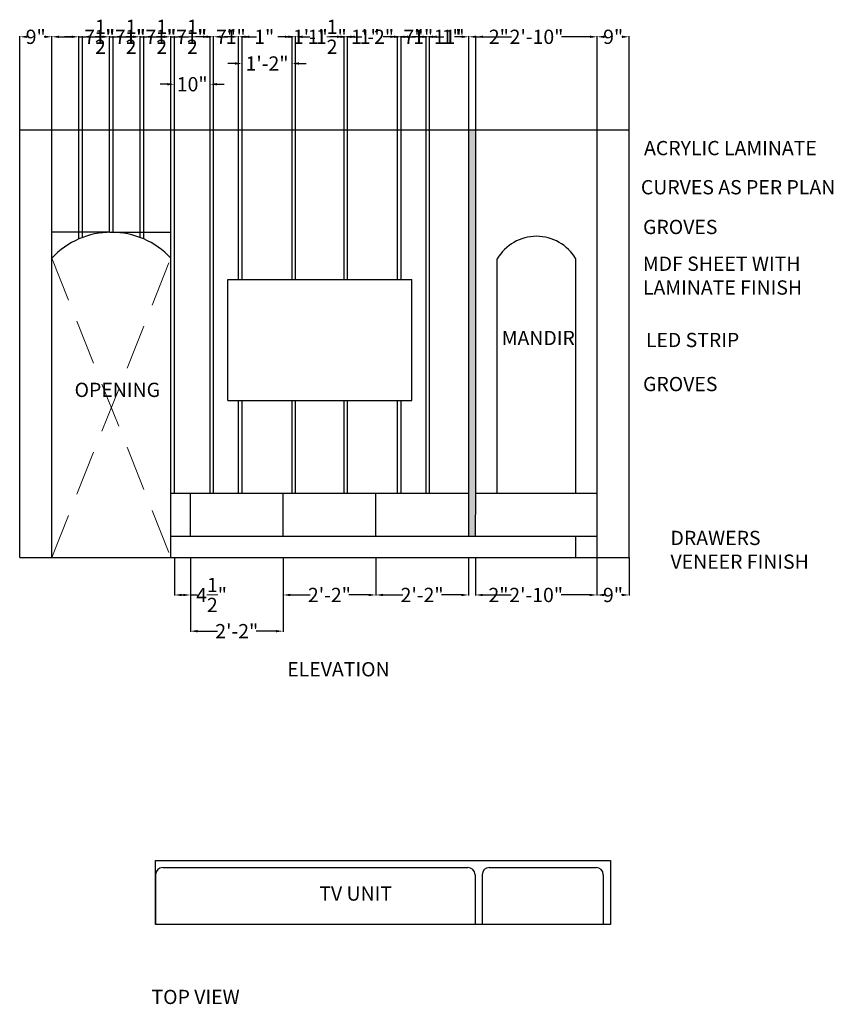
# Model space of a CAD drawing. Units: inches. Extents: x 114 to 342, y 174 to 451.
import ezdxf

# ---------------------------------------------------------------- set-up
doc = ezdxf.new("R2010")
doc.units = ezdxf.units.IN
doc.header["$MEASUREMENT"] = 0
doc.linetypes.add('DASHED', pattern=[19.05, 12.7, -6.35])
for name, color, linetype, lineweight in [('A-ANNO-DIMS', 2, 'Continuous', 18), ('A-ANNO-TEXT', 3, 'Continuous', 18), ('A-ELEV', 7, 'Continuous', 25), ('A-ELEV-OPNG', 8, 'DASHED', 18), ('A-ELEV-PATT', 8, 'Continuous', 13), ('A-FURN', 7, 'Continuous', 25)]:
    doc.layers.add(name, color=color, linetype=linetype, lineweight=lineweight)
doc.styles.get("Standard").update_dxf_attribs({"font": 'arial.ttf'})
doc.dimstyles.get("Standard").update_dxf_attribs({"dimtxt": 4, "dimasz": 2, "dimexe": 0.18, "dimexo": 0.0625, "dimgap": 0.09, "dimtad": 0, "dimtih": 1, "dimtoh": 1, "dimdec": 1, "dimzin": 0, "dimdsep": 46, "dimlunit": 4, "dimtxsty": 'Standard', "dimcen": 0.09, "dimadec": 0, "dimazin": 0, "dimtfac": 1, "dimtdec": 1, "dimtofl": 0, "dimtmove": 0, "dimatfit": 3, "dimfxl": 1, "dimtolj": 1, "dimtzin": 0, "dimarcsym": 1})

# ---------------------------------------------------------------- blocks, each defined once
blk = doc.blocks.new('*D1')
at = {"layer": 'A-ANNO-DIMS', "color": 0, "lineweight": -2, "transparency": 16777216}
for p, q in [((114.04, 419.84), (114.04, 446.03)), ((116.04, 445.85), (116.15, 445.85)), ((121.04, 445.85), (120.93, 445.85)), ((123.04, 419.84), (123.04, 446.03))]:
    blk.add_line(p, q, dxfattribs=at)
at = {"layer": 'A-ANNO-DIMS', "color": 0, "transparency": 16777216}
for points in [[(116.04, 446.18), (116.04, 445.52), (114.04, 445.85)], [(121.04, 446.18), (121.04, 445.52), (123.04, 445.85)]]:
    blk.add_solid(points, dxfattribs=at)
at = {"layer": 'Defpoints', "color": 0, "transparency": 16777216}
for p in [(123.04, 445.85), (114.04, 419.78), (123.04, 419.78)]:
    blk.add_point(p, dxfattribs=at)
at = {"layer": 'A-ANNO-DIMS', "color": 0, "transparency": 16777216, "insert": (118.54, 445.85), "char_height": 4, "attachment_point": 5}
blk.add_mtext('\\A1;9"', dxfattribs=at)
blk = doc.blocks.new('*D2')
at = {"layer": 'A-ANNO-DIMS', "color": 0, "lineweight": -2, "transparency": 16777216}
for p, q in [((123.04, 419.84), (123.04, 446.03)), ((125.04, 445.85), (128.64, 445.85)), ((130.64, 419.84), (130.64, 446.03)), ((130.64, 445.85), (132.64, 445.85))]:
    blk.add_line(p, q, dxfattribs=at)
at = {"layer": 'A-ANNO-DIMS', "color": 0, "transparency": 16777216}
for points in [[(125.04, 446.18), (125.04, 445.52), (123.04, 445.85)], [(128.64, 446.18), (128.64, 445.52), (130.64, 445.85)]]:
    blk.add_solid(points, dxfattribs=at)
at = {"layer": 'Defpoints', "color": 0, "transparency": 16777216}
for p in [(130.64, 445.85), (123.04, 419.78), (130.64, 419.78)]:
    blk.add_point(p, dxfattribs=at)
at = {"layer": 'A-ANNO-DIMS', "color": 0, "transparency": 16777216, "insert": (136.47, 445.85), "char_height": 4, "attachment_point": 5}
blk.add_mtext('\\A1;7{\\H1x;\\S1/2;}"', dxfattribs=at)
blk = doc.blocks.new('*D3')
at = {"layer": 'A-ANNO-DIMS', "color": 0, "lineweight": -2, "transparency": 16777216}
for p, q in [((128.64, 445.85), (126.64, 445.85)), ((130.64, 419.84), (130.64, 446.03)), ((131.64, 419.84), (131.64, 446.03)), ((133.64, 445.85), (135.64, 445.85))]:
    blk.add_line(p, q, dxfattribs=at)
at = {"layer": 'A-ANNO-DIMS', "color": 0, "transparency": 16777216}
for points in [[(128.64, 446.18), (128.64, 445.52), (130.64, 445.85)], [(133.64, 446.18), (133.64, 445.52), (131.64, 445.85)]]:
    blk.add_solid(points, dxfattribs=at)
at = {"layer": 'Defpoints', "color": 0, "transparency": 16777216}
for p in [(131.64, 445.85), (130.64, 419.78), (131.64, 419.78)]:
    blk.add_point(p, dxfattribs=at)
at = {"layer": 'A-ANNO-DIMS', "color": 0, "transparency": 16777216, "insert": (137.84, 445.85), "char_height": 4, "attachment_point": 5}
blk.add_mtext('\\A1;1"', dxfattribs=at)
blk = doc.blocks.new('*D4')
at = {"layer": 'A-ANNO-DIMS', "color": 0, "lineweight": -2, "transparency": 16777216}
for p, q in [((131.64, 419.84), (131.64, 446.03)), ((133.64, 445.85), (137.24, 445.85)), ((139.24, 419.84), (139.24, 446.03)), ((139.24, 445.85), (141.24, 445.85))]:
    blk.add_line(p, q, dxfattribs=at)
at = {"layer": 'A-ANNO-DIMS', "color": 0, "transparency": 16777216}
for points in [[(133.64, 446.18), (133.64, 445.52), (131.64, 445.85)], [(137.24, 446.18), (137.24, 445.52), (139.24, 445.85)]]:
    blk.add_solid(points, dxfattribs=at)
at = {"layer": 'Defpoints', "color": 0, "transparency": 16777216}
for p in [(139.24, 445.85), (131.64, 419.78), (139.24, 419.78)]:
    blk.add_point(p, dxfattribs=at)
at = {"layer": 'A-ANNO-DIMS', "color": 0, "transparency": 16777216, "insert": (145.07, 445.85), "char_height": 4, "attachment_point": 5}
blk.add_mtext('\\A1;7{\\H1x;\\S1/2;}"', dxfattribs=at)
blk = doc.blocks.new('*D5')
at = {"layer": 'A-ANNO-DIMS', "color": 0, "lineweight": -2, "transparency": 16777216}
for p, q in [((137.24, 445.85), (135.24, 445.85)), ((139.24, 419.84), (139.24, 446.03)), ((140.24, 419.84), (140.24, 446.03)), ((142.24, 445.85), (144.24, 445.85))]:
    blk.add_line(p, q, dxfattribs=at)
at = {"layer": 'A-ANNO-DIMS', "color": 0, "transparency": 16777216}
for points in [[(137.24, 446.18), (137.24, 445.52), (139.24, 445.85)], [(142.24, 446.18), (142.24, 445.52), (140.24, 445.85)]]:
    blk.add_solid(points, dxfattribs=at)
at = {"layer": 'Defpoints', "color": 0, "transparency": 16777216}
for p in [(140.24, 445.85), (139.24, 419.78), (140.24, 419.78)]:
    blk.add_point(p, dxfattribs=at)
at = {"layer": 'A-ANNO-DIMS', "color": 0, "transparency": 16777216, "insert": (146.44, 445.85), "char_height": 4, "attachment_point": 5}
blk.add_mtext('\\A1;1"', dxfattribs=at)
blk = doc.blocks.new('*D6')
at = {"layer": 'A-ANNO-DIMS', "color": 0, "lineweight": -2, "transparency": 16777216}
for p, q in [((140.24, 419.84), (140.24, 446.03)), ((142.24, 445.85), (145.84, 445.85)), ((147.84, 419.84), (147.84, 446.03)), ((147.84, 445.85), (149.84, 445.85))]:
    blk.add_line(p, q, dxfattribs=at)
at = {"layer": 'A-ANNO-DIMS', "color": 0, "transparency": 16777216}
for points in [[(142.24, 446.18), (142.24, 445.52), (140.24, 445.85)], [(145.84, 446.18), (145.84, 445.52), (147.84, 445.85)]]:
    blk.add_solid(points, dxfattribs=at)
at = {"layer": 'Defpoints', "color": 0, "transparency": 16777216}
for p in [(147.84, 445.85), (140.24, 419.78), (147.84, 419.78)]:
    blk.add_point(p, dxfattribs=at)
at = {"layer": 'A-ANNO-DIMS', "color": 0, "transparency": 16777216, "insert": (153.67, 445.85), "char_height": 4, "attachment_point": 5}
blk.add_mtext('\\A1;7{\\H1x;\\S1/2;}"', dxfattribs=at)
blk = doc.blocks.new('*D7')
at = {"layer": 'A-ANNO-DIMS', "color": 0, "lineweight": -2, "transparency": 16777216}
for p, q in [((145.84, 445.85), (143.84, 445.85)), ((147.84, 419.84), (147.84, 446.03)), ((148.84, 419.84), (148.84, 446.03)), ((150.84, 445.85), (152.84, 445.85))]:
    blk.add_line(p, q, dxfattribs=at)
at = {"layer": 'A-ANNO-DIMS', "color": 0, "transparency": 16777216}
for points in [[(145.84, 446.18), (145.84, 445.52), (147.84, 445.85)], [(150.84, 446.18), (150.84, 445.52), (148.84, 445.85)]]:
    blk.add_solid(points, dxfattribs=at)
at = {"layer": 'Defpoints', "color": 0, "transparency": 16777216}
for p in [(148.84, 445.85), (147.84, 419.78), (148.84, 419.78)]:
    blk.add_point(p, dxfattribs=at)
at = {"layer": 'A-ANNO-DIMS', "color": 0, "transparency": 16777216, "insert": (155.04, 445.85), "char_height": 4, "attachment_point": 5}
blk.add_mtext('\\A1;1"', dxfattribs=at)
blk = doc.blocks.new('*D8')
at = {"layer": 'A-ANNO-DIMS', "color": 0, "lineweight": -2, "transparency": 16777216}
for p, q in [((148.84, 419.84), (148.84, 446.03)), ((150.84, 445.85), (154.44, 445.85)), ((156.44, 419.84), (156.44, 446.03)), ((156.44, 445.85), (158.44, 445.85))]:
    blk.add_line(p, q, dxfattribs=at)
at = {"layer": 'A-ANNO-DIMS', "color": 0, "transparency": 16777216}
for points in [[(150.84, 446.18), (150.84, 445.52), (148.84, 445.85)], [(154.44, 446.18), (154.44, 445.52), (156.44, 445.85)]]:
    blk.add_solid(points, dxfattribs=at)
at = {"layer": 'Defpoints', "color": 0, "transparency": 16777216}
for p in [(156.44, 445.85), (148.84, 419.78), (156.44, 419.78)]:
    blk.add_point(p, dxfattribs=at)
at = {"layer": 'A-ANNO-DIMS', "color": 0, "transparency": 16777216, "insert": (162.27, 445.85), "char_height": 4, "attachment_point": 5}
blk.add_mtext('\\A1;7{\\H1x;\\S1/2;}"', dxfattribs=at)
blk = doc.blocks.new('*D9')
at = {"layer": 'A-ANNO-DIMS', "color": 0, "lineweight": -2, "transparency": 16777216}
for p, q in [((154.44, 445.85), (152.44, 445.85)), ((156.44, 419.84), (156.44, 446.03)), ((157.44, 419.84), (157.44, 446.03)), ((159.44, 445.85), (161.44, 445.85))]:
    blk.add_line(p, q, dxfattribs=at)
at = {"layer": 'A-ANNO-DIMS', "color": 0, "transparency": 16777216}
for points in [[(154.44, 446.18), (154.44, 445.52), (156.44, 445.85)], [(159.44, 446.18), (159.44, 445.52), (157.44, 445.85)]]:
    blk.add_solid(points, dxfattribs=at)
at = {"layer": 'Defpoints', "color": 0, "transparency": 16777216}
for p in [(157.44, 445.85), (156.44, 419.78), (157.44, 419.78)]:
    blk.add_point(p, dxfattribs=at)
at = {"layer": 'A-ANNO-DIMS', "color": 0, "transparency": 16777216, "insert": (163.64, 445.85), "char_height": 4, "attachment_point": 5}
blk.add_mtext('\\A1;1"', dxfattribs=at)
blk = doc.blocks.new('*D10')
at = {"layer": 'A-ANNO-DIMS', "color": 0, "lineweight": -2, "transparency": 16777216}
for p, q in [((155.44, 432.55), (153.44, 432.55)), ((157.44, 406.53), (157.44, 432.73)), ((167.44, 406.53), (167.44, 432.73)), ((169.44, 432.55), (171.44, 432.55))]:
    blk.add_line(p, q, dxfattribs=at)
at = {"layer": 'A-ANNO-DIMS', "color": 0, "transparency": 16777216}
for points in [[(155.44, 432.88), (155.44, 432.21), (157.44, 432.55)], [(169.44, 432.88), (169.44, 432.21), (167.44, 432.55)]]:
    blk.add_solid(points, dxfattribs=at)
at = {"layer": 'Defpoints', "color": 0, "transparency": 16777216}
for p in [(167.44, 432.55), (157.44, 406.47), (167.44, 406.47)]:
    blk.add_point(p, dxfattribs=at)
at = {"layer": 'A-ANNO-DIMS', "color": 0, "transparency": 16777216, "insert": (162.44, 432.55), "char_height": 4, "attachment_point": 5}
blk.add_mtext('\\A1;10"', dxfattribs=at)
blk = doc.blocks.new('*D11')
at = {"layer": 'A-ANNO-DIMS', "color": 0, "lineweight": -2, "transparency": 16777216}
for p, q in [((165.44, 445.85), (163.44, 445.85)), ((167.44, 419.84), (167.44, 446.03)), ((168.44, 419.84), (168.44, 446.03)), ((170.44, 445.85), (172.44, 445.85))]:
    blk.add_line(p, q, dxfattribs=at)
at = {"layer": 'A-ANNO-DIMS', "color": 0, "transparency": 16777216}
for points in [[(165.44, 446.18), (165.44, 445.52), (167.44, 445.85)], [(170.44, 446.18), (170.44, 445.52), (168.44, 445.85)]]:
    blk.add_solid(points, dxfattribs=at)
at = {"layer": 'Defpoints', "color": 0, "transparency": 16777216}
for p in [(168.44, 445.85), (167.44, 419.78), (168.44, 419.78)]:
    blk.add_point(p, dxfattribs=at)
at = {"layer": 'A-ANNO-DIMS', "color": 0, "transparency": 16777216, "insert": (174.64, 445.85), "char_height": 4, "attachment_point": 5}
blk.add_mtext('\\A1;1"', dxfattribs=at)
blk = doc.blocks.new('*D12')
at = {"layer": 'A-ANNO-DIMS', "color": 0, "lineweight": -2, "transparency": 16777216}
for p, q in [((166.44, 445.85), (164.44, 445.85)), ((168.44, 419.84), (168.44, 446.03)), ((175.44, 419.84), (175.44, 446.03)), ((177.44, 445.85), (179.44, 445.85))]:
    blk.add_line(p, q, dxfattribs=at)
at = {"layer": 'A-ANNO-DIMS', "color": 0, "transparency": 16777216}
for points in [[(166.44, 446.18), (166.44, 445.52), (168.44, 445.85)], [(177.44, 446.18), (177.44, 445.52), (175.44, 445.85)]]:
    blk.add_solid(points, dxfattribs=at)
at = {"layer": 'Defpoints', "color": 0, "transparency": 16777216}
for p in [(175.44, 445.85), (168.44, 419.78), (175.44, 419.78)]:
    blk.add_point(p, dxfattribs=at)
at = {"layer": 'A-ANNO-DIMS', "color": 0, "transparency": 16777216, "insert": (171.94, 445.85), "char_height": 4, "attachment_point": 5}
blk.add_mtext('\\A1;7"', dxfattribs=at)
blk = doc.blocks.new('*D13')
at = {"layer": 'A-ANNO-DIMS', "color": 0, "lineweight": -2, "transparency": 16777216}
for p, q in [((173.44, 445.85), (171.44, 445.85)), ((175.44, 419.84), (175.44, 446.03)), ((176.44, 419.84), (176.44, 446.03)), ((178.44, 445.85), (180.44, 445.85))]:
    blk.add_line(p, q, dxfattribs=at)
at = {"layer": 'A-ANNO-DIMS', "color": 0, "transparency": 16777216}
for points in [[(173.44, 446.18), (173.44, 445.52), (175.44, 445.85)], [(178.44, 446.18), (178.44, 445.52), (176.44, 445.85)]]:
    blk.add_solid(points, dxfattribs=at)
at = {"layer": 'Defpoints', "color": 0, "transparency": 16777216}
for p in [(176.44, 445.85), (175.44, 419.78), (176.44, 419.78)]:
    blk.add_point(p, dxfattribs=at)
at = {"layer": 'A-ANNO-DIMS', "color": 0, "transparency": 16777216, "insert": (182.64, 445.85), "char_height": 4, "attachment_point": 5}
blk.add_mtext('\\A1;1"', dxfattribs=at)
blk = doc.blocks.new('*D14')
at = {"layer": 'A-ANNO-DIMS', "color": 0, "lineweight": -2, "transparency": 16777216}
for p, q in [((174.44, 438.36), (172.44, 438.36)), ((176.44, 412.35), (176.44, 438.54)), ((190.44, 412.35), (190.44, 438.54)), ((192.44, 438.36), (194.44, 438.36))]:
    blk.add_line(p, q, dxfattribs=at)
at = {"layer": 'A-ANNO-DIMS', "color": 0, "transparency": 16777216}
for points in [[(174.44, 438.7), (174.44, 438.03), (176.44, 438.36)], [(192.44, 438.7), (192.44, 438.03), (190.44, 438.36)]]:
    blk.add_solid(points, dxfattribs=at)
at = {"layer": 'Defpoints', "color": 0, "transparency": 16777216}
for p in [(190.44, 438.36), (176.44, 412.29), (190.44, 412.29)]:
    blk.add_point(p, dxfattribs=at)
at = {"layer": 'A-ANNO-DIMS', "color": 0, "transparency": 16777216, "insert": (183.44, 438.36), "char_height": 4, "attachment_point": 5}
blk.add_mtext('\\A1;1\'-2"', dxfattribs=at)
blk = doc.blocks.new('*D15')
at = {"layer": 'A-ANNO-DIMS', "color": 0, "lineweight": -2, "transparency": 16777216}
for p, q in [((188.44, 445.85), (186.44, 445.85)), ((190.44, 419.84), (190.44, 446.03)), ((191.44, 419.84), (191.44, 446.03)), ((193.44, 445.85), (195.44, 445.85))]:
    blk.add_line(p, q, dxfattribs=at)
at = {"layer": 'A-ANNO-DIMS', "color": 0, "transparency": 16777216}
for points in [[(188.44, 446.18), (188.44, 445.52), (190.44, 445.85)], [(193.44, 446.18), (193.44, 445.52), (191.44, 445.85)]]:
    blk.add_solid(points, dxfattribs=at)
at = {"layer": 'Defpoints', "color": 0, "transparency": 16777216}
for p in [(191.44, 445.85), (190.44, 419.78), (191.44, 419.78)]:
    blk.add_point(p, dxfattribs=at)
at = {"layer": 'A-ANNO-DIMS', "color": 0, "transparency": 16777216, "insert": (197.64, 445.85), "char_height": 4, "attachment_point": 5}
blk.add_mtext('\\A1;1"', dxfattribs=at)
blk = doc.blocks.new('*D16')
at = {"layer": 'A-ANNO-DIMS', "color": 0, "lineweight": -2, "transparency": 16777216}
for p, q in [((189.44, 445.85), (187.44, 445.85)), ((191.44, 419.84), (191.44, 446.03)), ((205.04, 419.84), (205.04, 446.03)), ((207.04, 445.85), (209.04, 445.85))]:
    blk.add_line(p, q, dxfattribs=at)
at = {"layer": 'A-ANNO-DIMS', "color": 0, "transparency": 16777216}
for points in [[(189.44, 446.18), (189.44, 445.52), (191.44, 445.85)], [(207.04, 446.18), (207.04, 445.52), (205.04, 445.85)]]:
    blk.add_solid(points, dxfattribs=at)
at = {"layer": 'Defpoints', "color": 0, "transparency": 16777216}
for p in [(205.04, 445.85), (191.44, 419.78), (205.04, 419.78)]:
    blk.add_point(p, dxfattribs=at)
at = {"layer": 'A-ANNO-DIMS', "color": 0, "transparency": 16777216, "insert": (198.24, 445.85), "char_height": 4, "attachment_point": 5}
blk.add_mtext('\\A1;1\'-1{\\H1x;\\S1/2;}"', dxfattribs=at)
blk = doc.blocks.new('*D17')
at = {"layer": 'A-ANNO-DIMS', "color": 0, "lineweight": -2, "transparency": 16777216}
for p, q in [((203.04, 445.85), (201.04, 445.85)), ((205.04, 419.84), (205.04, 446.03)), ((206.04, 419.84), (206.04, 446.03)), ((208.04, 445.85), (210.04, 445.85))]:
    blk.add_line(p, q, dxfattribs=at)
at = {"layer": 'A-ANNO-DIMS', "color": 0, "transparency": 16777216}
for points in [[(203.04, 446.18), (203.04, 445.52), (205.04, 445.85)], [(208.04, 446.18), (208.04, 445.52), (206.04, 445.85)]]:
    blk.add_solid(points, dxfattribs=at)
at = {"layer": 'Defpoints', "color": 0, "transparency": 16777216}
for p in [(206.04, 445.85), (205.04, 419.78), (206.04, 419.78)]:
    blk.add_point(p, dxfattribs=at)
at = {"layer": 'A-ANNO-DIMS', "color": 0, "transparency": 16777216, "insert": (212.24, 445.85), "char_height": 4, "attachment_point": 5}
blk.add_mtext('\\A1;1"', dxfattribs=at)
blk = doc.blocks.new('*D18')
at = {"layer": 'A-ANNO-DIMS', "color": 0, "lineweight": -2, "transparency": 16777216}
for p, q in [((204.04, 445.85), (202.04, 445.85)), ((206.04, 419.84), (206.04, 446.03)), ((220.04, 419.84), (220.04, 446.03)), ((222.04, 445.85), (224.04, 445.85))]:
    blk.add_line(p, q, dxfattribs=at)
at = {"layer": 'A-ANNO-DIMS', "color": 0, "transparency": 16777216}
for points in [[(204.04, 446.18), (204.04, 445.52), (206.04, 445.85)], [(222.04, 446.18), (222.04, 445.52), (220.04, 445.85)]]:
    blk.add_solid(points, dxfattribs=at)
at = {"layer": 'Defpoints', "color": 0, "transparency": 16777216}
for p in [(220.04, 445.85), (206.04, 419.78), (220.04, 419.78)]:
    blk.add_point(p, dxfattribs=at)
at = {"layer": 'A-ANNO-DIMS', "color": 0, "transparency": 16777216, "insert": (213.04, 445.85), "char_height": 4, "attachment_point": 5}
blk.add_mtext('\\A1;1\'-2"', dxfattribs=at)
blk = doc.blocks.new('*D19')
at = {"layer": 'A-ANNO-DIMS', "color": 0, "lineweight": -2, "transparency": 16777216}
for p, q in [((218.04, 445.85), (216.04, 445.85)), ((220.04, 419.84), (220.04, 446.03)), ((221.04, 419.84), (221.04, 446.03)), ((223.04, 445.85), (225.04, 445.85))]:
    blk.add_line(p, q, dxfattribs=at)
at = {"layer": 'A-ANNO-DIMS', "color": 0, "transparency": 16777216}
for points in [[(218.04, 446.18), (218.04, 445.52), (220.04, 445.85)], [(223.04, 446.18), (223.04, 445.52), (221.04, 445.85)]]:
    blk.add_solid(points, dxfattribs=at)
at = {"layer": 'Defpoints', "color": 0, "transparency": 16777216}
for p in [(221.04, 445.85), (220.04, 419.78), (221.04, 419.78)]:
    blk.add_point(p, dxfattribs=at)
at = {"layer": 'A-ANNO-DIMS', "color": 0, "transparency": 16777216, "insert": (227.24, 445.85), "char_height": 4, "attachment_point": 5}
blk.add_mtext('\\A1;1"', dxfattribs=at)
blk = doc.blocks.new('*D20')
at = {"layer": 'A-ANNO-DIMS', "color": 0, "lineweight": -2, "transparency": 16777216}
for p, q in [((219.04, 445.85), (217.04, 445.85)), ((221.04, 419.84), (221.04, 446.03)), ((228.04, 419.84), (228.04, 446.03)), ((230.04, 445.85), (232.04, 445.85))]:
    blk.add_line(p, q, dxfattribs=at)
at = {"layer": 'A-ANNO-DIMS', "color": 0, "transparency": 16777216}
for points in [[(219.04, 446.18), (219.04, 445.52), (221.04, 445.85)], [(230.04, 446.18), (230.04, 445.52), (228.04, 445.85)]]:
    blk.add_solid(points, dxfattribs=at)
at = {"layer": 'Defpoints', "color": 0, "transparency": 16777216}
for p in [(228.04, 445.85), (221.04, 419.78), (228.04, 419.78)]:
    blk.add_point(p, dxfattribs=at)
at = {"layer": 'A-ANNO-DIMS', "color": 0, "transparency": 16777216, "insert": (224.54, 445.85), "char_height": 4, "attachment_point": 5}
blk.add_mtext('\\A1;7"', dxfattribs=at)
blk = doc.blocks.new('*D21')
at = {"layer": 'A-ANNO-DIMS', "color": 0, "lineweight": -2, "transparency": 16777216}
for p, q in [((226.04, 445.85), (224.04, 445.85)), ((228.04, 419.84), (228.04, 446.03)), ((229.04, 419.84), (229.04, 446.03)), ((231.04, 445.85), (233.04, 445.85))]:
    blk.add_line(p, q, dxfattribs=at)
at = {"layer": 'A-ANNO-DIMS', "color": 0, "transparency": 16777216}
for points in [[(226.04, 446.18), (226.04, 445.52), (228.04, 445.85)], [(231.04, 446.18), (231.04, 445.52), (229.04, 445.85)]]:
    blk.add_solid(points, dxfattribs=at)
at = {"layer": 'Defpoints', "color": 0, "transparency": 16777216}
for p in [(229.04, 445.85), (228.04, 419.78), (229.04, 419.78)]:
    blk.add_point(p, dxfattribs=at)
at = {"layer": 'A-ANNO-DIMS', "color": 0, "transparency": 16777216, "insert": (235.24, 445.85), "char_height": 4, "attachment_point": 5}
blk.add_mtext('\\A1;1"', dxfattribs=at)
blk = doc.blocks.new('*D22')
at = {"layer": 'A-ANNO-DIMS', "color": 0, "lineweight": -2, "transparency": 16777216}
for p, q in [((227.04, 445.85), (225.04, 445.85)), ((229.04, 419.84), (229.04, 446.03)), ((240.04, 419.84), (240.04, 446.03)), ((242.04, 445.85), (244.04, 445.85))]:
    blk.add_line(p, q, dxfattribs=at)
at = {"layer": 'A-ANNO-DIMS', "color": 0, "transparency": 16777216}
for points in [[(227.04, 446.18), (227.04, 445.52), (229.04, 445.85)], [(242.04, 446.18), (242.04, 445.52), (240.04, 445.85)]]:
    blk.add_solid(points, dxfattribs=at)
at = {"layer": 'Defpoints', "color": 0, "transparency": 16777216}
for p in [(240.04, 445.85), (229.04, 419.78), (240.04, 419.78)]:
    blk.add_point(p, dxfattribs=at)
at = {"layer": 'A-ANNO-DIMS', "color": 0, "transparency": 16777216, "insert": (234.54, 445.85), "char_height": 4, "attachment_point": 5}
blk.add_mtext('\\A1;11"', dxfattribs=at)
blk = doc.blocks.new('*D23')
at = {"layer": 'A-ANNO-DIMS', "color": 0, "lineweight": -2, "transparency": 16777216}
for p, q in [((238.04, 445.85), (236.04, 445.85)), ((240.04, 419.84), (240.04, 446.03)), ((242.04, 419.84), (242.04, 446.03)), ((244.04, 445.85), (246.04, 445.85))]:
    blk.add_line(p, q, dxfattribs=at)
at = {"layer": 'A-ANNO-DIMS', "color": 0, "transparency": 16777216}
for points in [[(238.04, 446.18), (238.04, 445.52), (240.04, 445.85)], [(244.04, 446.18), (244.04, 445.52), (242.04, 445.85)]]:
    blk.add_solid(points, dxfattribs=at)
at = {"layer": 'Defpoints', "color": 0, "transparency": 16777216}
for p in [(242.04, 445.85), (240.04, 419.78), (242.04, 419.78)]:
    blk.add_point(p, dxfattribs=at)
at = {"layer": 'A-ANNO-DIMS', "color": 0, "transparency": 16777216, "insert": (248.47, 445.85), "char_height": 4, "attachment_point": 5}
blk.add_mtext('\\A1;2"', dxfattribs=at)
blk = doc.blocks.new('*D24')
at = {"layer": 'A-ANNO-DIMS', "color": 0, "lineweight": -2, "transparency": 16777216}
for p, q in [((242.04, 419.84), (242.04, 446.03)), ((244.04, 445.85), (252.05, 445.85)), ((274.04, 445.85), (266.04, 445.85)), ((276.04, 419.84), (276.04, 446.03))]:
    blk.add_line(p, q, dxfattribs=at)
at = {"layer": 'A-ANNO-DIMS', "color": 0, "transparency": 16777216}
for points in [[(244.04, 446.18), (244.04, 445.52), (242.04, 445.85)], [(274.04, 446.18), (274.04, 445.52), (276.04, 445.85)]]:
    blk.add_solid(points, dxfattribs=at)
at = {"layer": 'Defpoints', "color": 0, "transparency": 16777216}
for p in [(276.04, 445.85), (242.04, 419.78), (276.04, 419.78)]:
    blk.add_point(p, dxfattribs=at)
at = {"layer": 'A-ANNO-DIMS', "color": 0, "transparency": 16777216, "insert": (259.04, 445.85), "char_height": 4, "attachment_point": 5}
blk.add_mtext('\\A1;2\'-10"', dxfattribs=at)
blk = doc.blocks.new('*D25')
at = {"layer": 'A-ANNO-DIMS', "color": 0, "lineweight": -2, "transparency": 16777216}
for p, q in [((276.04, 419.84), (276.04, 446.03)), ((278.04, 445.85), (278.15, 445.85)), ((283.04, 445.85), (282.93, 445.85)), ((285.04, 419.84), (285.04, 446.03))]:
    blk.add_line(p, q, dxfattribs=at)
at = {"layer": 'A-ANNO-DIMS', "color": 0, "transparency": 16777216}
for points in [[(278.04, 446.18), (278.04, 445.52), (276.04, 445.85)], [(283.04, 446.18), (283.04, 445.52), (285.04, 445.85)]]:
    blk.add_solid(points, dxfattribs=at)
at = {"layer": 'Defpoints', "color": 0, "transparency": 16777216}
for p in [(285.04, 445.85), (276.04, 419.78), (285.04, 419.78)]:
    blk.add_point(p, dxfattribs=at)
at = {"layer": 'A-ANNO-DIMS', "color": 0, "transparency": 16777216, "insert": (280.54, 445.85), "char_height": 4, "attachment_point": 5}
blk.add_mtext('\\A1;9"', dxfattribs=at)
blk = doc.blocks.new('*D26')
at = {"layer": 'A-ANNO-DIMS', "color": 0, "lineweight": -2, "transparency": 16777216}
for p, q in [((157.44, 299.71), (157.44, 289.06)), ((161.94, 299.71), (161.94, 289.06)), ((159.44, 289.24), (159.94, 289.24)), ((161.94, 289.24), (163.94, 289.24))]:
    blk.add_line(p, q, dxfattribs=at)
at = {"layer": 'A-ANNO-DIMS', "color": 0, "transparency": 16777216}
for points in [[(159.44, 289.57), (159.44, 288.91), (157.44, 289.24)], [(159.94, 289.57), (159.94, 288.91), (161.94, 289.24)]]:
    blk.add_solid(points, dxfattribs=at)
at = {"layer": 'Defpoints', "color": 0, "transparency": 16777216}
for p in [(157.44, 299.78), (161.94, 299.78), (161.94, 289.24)]:
    blk.add_point(p, dxfattribs=at)
at = {"layer": 'A-ANNO-DIMS', "color": 0, "transparency": 16777216, "insert": (167.87, 289.24), "char_height": 4, "attachment_point": 5}
blk.add_mtext('\\A1;4{\\H1x;\\S1/2;}"', dxfattribs=at)
blk = doc.blocks.new('*D27')
at = {"layer": 'A-ANNO-DIMS', "color": 0, "lineweight": -2, "transparency": 16777216}
for p, q in [((161.94, 289.56), (161.94, 278.91)), ((187.94, 289.56), (187.94, 278.91)), ((163.94, 279.09), (169.5, 279.09)), ((185.94, 279.09), (180.38, 279.09))]:
    blk.add_line(p, q, dxfattribs=at)
at = {"layer": 'A-ANNO-DIMS', "color": 0, "transparency": 16777216}
for points in [[(163.94, 279.42), (163.94, 278.75), (161.94, 279.09)], [(185.94, 279.42), (185.94, 278.75), (187.94, 279.09)]]:
    blk.add_solid(points, dxfattribs=at)
at = {"layer": 'Defpoints', "color": 0, "transparency": 16777216}
for p in [(161.94, 289.62), (187.94, 289.62), (187.94, 279.09)]:
    blk.add_point(p, dxfattribs=at)
at = {"layer": 'A-ANNO-DIMS', "color": 0, "transparency": 16777216, "insert": (174.94, 279.09), "char_height": 4, "attachment_point": 5}
blk.add_mtext('\\A1;2\'-2"', dxfattribs=at)
blk = doc.blocks.new('*D28')
at = {"layer": 'A-ANNO-DIMS', "color": 0, "lineweight": -2, "transparency": 16777216}
for p, q in [((187.94, 299.71), (187.94, 289.06)), ((213.94, 299.71), (213.94, 289.06)), ((189.94, 289.24), (195.5, 289.24)), ((211.94, 289.24), (206.38, 289.24))]:
    blk.add_line(p, q, dxfattribs=at)
at = {"layer": 'A-ANNO-DIMS', "color": 0, "transparency": 16777216}
for points in [[(189.94, 289.57), (189.94, 288.91), (187.94, 289.24)], [(211.94, 289.57), (211.94, 288.91), (213.94, 289.24)]]:
    blk.add_solid(points, dxfattribs=at)
at = {"layer": 'Defpoints', "color": 0, "transparency": 16777216}
for p in [(187.94, 299.78), (213.94, 299.78), (213.94, 289.24)]:
    blk.add_point(p, dxfattribs=at)
at = {"layer": 'A-ANNO-DIMS', "color": 0, "transparency": 16777216, "insert": (200.94, 289.24), "char_height": 4, "attachment_point": 5}
blk.add_mtext('\\A1;2\'-2"', dxfattribs=at)
blk = doc.blocks.new('*D29')
at = {"layer": 'A-ANNO-DIMS', "color": 0, "lineweight": -2, "transparency": 16777216}
for p, q in [((213.94, 299.71), (213.94, 289.06)), ((239.94, 299.71), (239.94, 289.06)), ((215.94, 289.24), (221.5, 289.24)), ((237.94, 289.24), (232.38, 289.24))]:
    blk.add_line(p, q, dxfattribs=at)
at = {"layer": 'A-ANNO-DIMS', "color": 0, "transparency": 16777216}
for points in [[(215.94, 289.57), (215.94, 288.91), (213.94, 289.24)], [(237.94, 289.57), (237.94, 288.91), (239.94, 289.24)]]:
    blk.add_solid(points, dxfattribs=at)
at = {"layer": 'Defpoints', "color": 0, "transparency": 16777216}
for p in [(213.94, 299.78), (239.94, 299.78), (239.94, 289.24)]:
    blk.add_point(p, dxfattribs=at)
at = {"layer": 'A-ANNO-DIMS', "color": 0, "transparency": 16777216, "insert": (226.94, 289.24), "char_height": 4, "attachment_point": 5}
blk.add_mtext('\\A1;2\'-2"', dxfattribs=at)
blk = doc.blocks.new('*D30')
at = {"layer": 'A-ANNO-DIMS', "color": 0, "lineweight": -2, "transparency": 16777216}
for p, q in [((239.94, 299.71), (239.94, 289.06)), ((241.94, 299.71), (241.94, 289.06)), ((237.94, 289.24), (235.94, 289.24)), ((243.94, 289.24), (245.94, 289.24))]:
    blk.add_line(p, q, dxfattribs=at)
at = {"layer": 'A-ANNO-DIMS', "color": 0, "transparency": 16777216}
for points in [[(237.94, 289.57), (237.94, 288.91), (239.94, 289.24)], [(243.94, 289.57), (243.94, 288.91), (241.94, 289.24)]]:
    blk.add_solid(points, dxfattribs=at)
at = {"layer": 'Defpoints', "color": 0, "transparency": 16777216}
for p in [(239.94, 299.78), (241.94, 299.78), (241.94, 289.24)]:
    blk.add_point(p, dxfattribs=at)
at = {"layer": 'A-ANNO-DIMS', "color": 0, "transparency": 16777216, "insert": (248.37, 289.24), "char_height": 4, "attachment_point": 5}
blk.add_mtext('\\A1;2"', dxfattribs=at)
blk = doc.blocks.new('*D31')
at = {"layer": 'A-ANNO-DIMS', "color": 0, "lineweight": -2, "transparency": 16777216}
for p, q in [((241.94, 299.71), (241.94, 289.06)), ((275.94, 299.71), (275.94, 289.06)), ((243.94, 289.24), (251.95, 289.24)), ((273.94, 289.24), (265.94, 289.24))]:
    blk.add_line(p, q, dxfattribs=at)
at = {"layer": 'A-ANNO-DIMS', "color": 0, "transparency": 16777216}
for points in [[(243.94, 289.57), (243.94, 288.91), (241.94, 289.24)], [(273.94, 289.57), (273.94, 288.91), (275.94, 289.24)]]:
    blk.add_solid(points, dxfattribs=at)
at = {"layer": 'Defpoints', "color": 0, "transparency": 16777216}
for p in [(241.94, 299.78), (275.94, 299.78), (275.94, 289.24)]:
    blk.add_point(p, dxfattribs=at)
at = {"layer": 'A-ANNO-DIMS', "color": 0, "transparency": 16777216, "insert": (258.94, 289.24), "char_height": 4, "attachment_point": 5}
blk.add_mtext('\\A1;2\'-10"', dxfattribs=at)
blk = doc.blocks.new('*D32')
at = {"layer": 'A-ANNO-DIMS', "color": 0, "lineweight": -2, "transparency": 16777216}
for p, q in [((275.94, 299.71), (275.94, 289.06)), ((285.04, 299.71), (285.04, 289.06)), ((277.94, 289.24), (278.1, 289.24)), ((283.04, 289.24), (282.88, 289.24))]:
    blk.add_line(p, q, dxfattribs=at)
at = {"layer": 'A-ANNO-DIMS', "color": 0, "transparency": 16777216}
for points in [[(277.94, 289.57), (277.94, 288.91), (275.94, 289.24)], [(283.04, 289.57), (283.04, 288.91), (285.04, 289.24)]]:
    blk.add_solid(points, dxfattribs=at)
at = {"layer": 'Defpoints', "color": 0, "transparency": 16777216}
for p in [(275.94, 299.78), (285.04, 299.78), (285.04, 289.24)]:
    blk.add_point(p, dxfattribs=at)
at = {"layer": 'A-ANNO-DIMS', "color": 0, "transparency": 16777216, "insert": (280.49, 289.24), "char_height": 4, "attachment_point": 5}
blk.add_mtext('\\A1;9"', dxfattribs=at)

msp = doc.modelspace()

# ---------------------------------------------------------------- hatches: boundary and pattern name
at = {"layer": 'A-ELEV-PATT'}
h = msp.add_hatch(color=256, dxfattribs=at)
h.dxf.hatch_style = 1
h.paths.add_polyline_path([(242.04, 419.78), (240.04, 419.78), (240.04, 305.78), (241.94, 305.78), (242.04, 317.78)])

# ---------------------------------------------------------------- linework, layer by layer
at = {"layer": 'A-ELEV'}
for p, q in [((114.04, 299.78), (114.04, 419.78)), ((114.04, 419.78), (123.04, 419.78)), ((123.04, 419.78), (130.64, 419.78)), ((123.04, 299.78), (123.04, 419.78)), ((130.64, 419.78), (131.64, 419.78)), ((130.64, 389.13), (130.64, 419.78)), ((131.64, 419.78), (139.24, 419.78)), ((131.64, 389.54), (131.64, 419.78)), ((139.24, 419.78), (140.24, 419.78)), ((139.24, 391.01), (139.24, 419.78)), ((140.24, 419.78), (147.84, 419.78)), ((140.24, 391.01), (140.24, 419.78)), ((147.84, 419.78), (148.84, 419.78)), ((147.84, 389.54), (147.84, 419.78)), ((148.84, 419.78), (156.44, 419.78)), ((148.84, 389.13), (148.84, 419.78)), ((156.44, 419.78), (157.44, 419.78)), ((156.44, 299.78), (156.44, 419.78)), ((157.44, 419.78), (167.44, 419.78)), ((157.44, 317.78), (157.44, 419.78)), ((167.44, 419.78), (168.44, 419.78)), ((167.44, 317.78), (167.44, 419.78)), ((168.44, 419.78), (175.44, 419.78)), ((168.44, 317.78), (168.44, 419.78)), ((175.44, 419.78), (176.44, 419.78)), ((175.44, 377.78), (175.44, 419.78)), ((176.44, 419.78), (190.44, 419.78)), ((176.44, 377.78), (176.44, 419.78)), ((190.44, 419.78), (191.44, 419.78)), ((190.44, 377.78), (190.44, 419.78)), ((191.44, 419.78), (205.04, 419.78)), ((191.44, 377.78), (191.44, 419.78)), ((205.04, 419.78), (206.04, 419.78)), ((205.04, 377.78), (205.04, 419.78)), ((206.04, 419.78), (220.04, 419.78)), ((206.04, 377.78), (206.04, 419.78)), ((220.04, 419.78), (221.04, 419.78)), ((220.04, 377.78), (220.04, 419.78)), ((221.04, 419.78), (228.04, 419.78)), ((221.04, 377.78), (221.04, 419.78)), ((228.04, 419.78), (229.04, 419.78)), ((228.04, 317.78), (228.04, 419.78)), ((229.04, 419.78), (240.04, 419.78)), ((229.04, 317.78), (229.04, 419.78)), ((240.04, 419.78), (242.04, 419.78)), ((240.04, 305.78), (240.04, 419.78)), ((242.04, 419.78), (276.04, 419.78)), ((242.04, 317.78), (242.04, 419.78)), ((276.04, 419.78), (285.04, 419.78)), ((276.04, 299.78), (276.04, 419.78)), ((285.04, 299.78), (285.04, 419.78)), ((139.24, 391.01), (123.04, 391.01)), ((139.24, 391.01), (156.44, 391.01)), ((248.04, 317.78), (248.04, 383.55)), ((270.04, 317.78), (270.04, 383.55)), ((172.44, 343.78), (172.44, 377.78)), ((172.44, 377.78), (224.04, 377.78)), ((224.04, 343.78), (224.04, 377.78)), ((172.44, 343.78), (224.04, 343.78)), ((175.44, 317.78), (175.44, 343.78)), ((176.44, 317.78), (176.44, 343.78)), ((190.44, 317.78), (190.44, 343.78)), ((191.44, 317.78), (191.44, 343.78)), ((205.04, 317.78), (205.04, 343.78)), ((206.04, 317.78), (206.04, 343.78)), ((220.04, 317.78), (220.04, 343.78)), ((221.04, 317.78), (221.04, 343.78)), ((156.44, 317.78), (161.94, 317.78)), ((161.94, 317.78), (187.94, 317.78)), ((161.94, 305.78), (161.94, 317.78)), ((187.94, 317.78), (213.94, 317.78)), ((187.94, 305.78), (187.94, 317.78)), ((213.94, 317.78), (239.94, 317.78)), ((213.94, 305.78), (213.94, 317.78)), ((239.94, 317.78), (240.04, 317.78)), ((241.94, 305.78), (242.04, 317.78)), ((242.04, 317.78), (275.94, 317.78)), ((156.44, 305.78), (161.94, 305.78)), ((161.94, 305.78), (187.94, 305.78)), ((187.94, 305.78), (213.94, 305.78)), ((213.94, 305.78), (239.94, 305.78)), ((239.94, 305.78), (241.94, 305.78)), ((241.94, 305.78), (275.94, 305.78)), ((247.94, 305.73), (247.94, 305.78)), ((270.04, 299.78), (270.04, 305.78)), ((114.04, 299.78), (123.04, 299.78)), ((123.04, 299.78), (157.44, 299.78)), ((157.44, 299.78), (161.94, 299.78)), ((161.94, 299.78), (187.94, 299.78)), ((187.94, 299.78), (213.94, 299.78)), ((213.94, 299.78), (239.94, 299.78)), ((239.94, 299.78), (241.94, 299.78)), ((241.94, 299.78), (275.94, 299.78)), ((275.94, 299.78), (285.04, 299.78))]:
    msp.add_line(p, q, dxfattribs=at)
for centre, radius, start, end in [((139.74, 368.14), 22.87, 43.1084, 136.8916), ((259.04, 377.14), 12.73, 30.2508, 149.7492)]:
    msp.add_arc(centre, radius, start, end, dxfattribs=at)
at = {"layer": 'A-ELEV-OPNG'}
for p, q in [((123.04, 383.78), (156.44, 299.78)), ((123.04, 299.78), (156.44, 383.78))]:
    msp.add_line(p, q, dxfattribs=at)
at = {"layer": 'A-FURN'}
for p, q in [((152.18, 214.76), (279.78, 214.76)), ((152.18, 196.76), (152.18, 214.76)), ((154.18, 212.76), (239.78, 212.76)), ((245.78, 212.76), (275.78, 212.76)), ((279.78, 214.76), (279.78, 202.76)), ((152.18, 210.76), (152.18, 196.76)), ((241.78, 210.76), (241.78, 196.76)), ((243.78, 210.76), (243.78, 196.76)), ((277.78, 210.76), (277.78, 202.76)), ((277.78, 202.76), (277.78, 196.76)), ((279.78, 202.76), (279.78, 196.76)), ((279.78, 196.76), (152.18, 196.76))]:
    msp.add_line(p, q, dxfattribs=at)
for centre, start, end in [((154.18, 210.76), 90, 180), ((239.78, 210.76), 0, 90), ((245.78, 210.76), 90, 180), ((275.78, 210.76), 0, 90)]:
    msp.add_arc(centre, 2, start, end, dxfattribs=at)

# ---------------------------------------------------------------- texts
at = {"layer": 'A-ANNO-TEXT', "char_height": 4, "attachment_point": 1}
for s, width, insert in [('ACRYLIC LAMINATE', 123.9342, (289.2, 416.63)), ('CURVES AS PER PLAN', 66.7735, (288.32, 405.65)), ('GROVES', 61.7729, (288.92, 394.5)), ('MDF SHEET WITH \\PLAMINATE FINISH', 94.2955, (288.89, 384.18)), ('MANDIR', 19.1737, (249.28, 363.34)), ('LED STRIP', 60.3384, (289.72, 362.78)), ('\\pxqc;OPENING', 32.198, (125.33, 348.79)), ('GROVES', 61.7729, (288.92, 350.42)), ('DRAWERS \\PVENEER FINISH', 122.7835, (296.63, 307.25)), ('\\pxqc;ELEVATION', 68.9218, (169.01, 270.4)), ('\\pxqc;TV UNIT', 45.8642, (185.36, 207.48)), ('TOP VIEW', 83.8579, (151.02, 178.46))]:
    msp.add_mtext_dynamic_manual_height_columns(s, width=width, gutter_width=20, heights=[0], dxfattribs=dict(at, insert=insert))

# ---------------------------------------------------------------- dimensions: what is measured, and where the dimension line sits
at = {"layer": 'A-ANNO-DIMS'}
for base, p1, p2, picture, middle in [((130.64, 445.85), (123.04, 419.78), (130.64, 419.78), '*D2', (136.47, 445.85)), ((139.24, 445.85), (131.64, 419.78), (139.24, 419.78), '*D4', (145.07, 445.85)), ((147.84, 445.85), (140.24, 419.78), (147.84, 419.78), '*D6', (153.67, 445.85)), ((156.44, 445.85), (148.84, 419.78), (156.44, 419.78), '*D8', (162.27, 445.85)), ((205.04, 445.85), (191.44, 419.78), (205.04, 419.78), '*D16', (198.24, 445.85)), ((123.04, 445.85), (114.04, 419.78), (123.04, 419.78), '*D1', (118.54, 445.85)), ((131.64, 445.85), (130.64, 419.78), (131.64, 419.78), '*D3', (137.84, 445.85)), ((140.24, 445.85), (139.24, 419.78), (140.24, 419.78), '*D5', (146.44, 445.85)), ((148.84, 445.85), (147.84, 419.78), (148.84, 419.78), '*D7', (155.04, 445.85)), ((157.44, 445.85), (156.44, 419.78), (157.44, 419.78), '*D9', (163.64, 445.85)), ((168.44, 445.85), (167.44, 419.78), (168.44, 419.78), '*D11', (174.64, 445.85)), ((175.44, 445.85), (168.44, 419.78), (175.44, 419.78), '*D12', (171.94, 445.85)), ((176.44, 445.85), (175.44, 419.78), (176.44, 419.78), '*D13', (182.64, 445.85)), ((191.44, 445.85), (190.44, 419.78), (191.44, 419.78), '*D15', (197.64, 445.85)), ((206.04, 445.85), (205.04, 419.78), (206.04, 419.78), '*D17', (212.24, 445.85)), ((220.04, 445.85), (206.04, 419.78), (220.04, 419.78), '*D18', (213.04, 445.85)), ((221.04, 445.85), (220.04, 419.78), (221.04, 419.78), '*D19', (227.24, 445.85)), ((228.04, 445.85), (221.04, 419.78), (228.04, 419.78), '*D20', (224.54, 445.85)), ((229.04, 445.85), (228.04, 419.78), (229.04, 419.78), '*D21', (235.24, 445.85)), ((240.04, 445.85), (229.04, 419.78), (240.04, 419.78), '*D22', (234.54, 445.85)), ((242.04, 445.85), (240.04, 419.78), (242.04, 419.78), '*D23', (248.47, 445.85)), ((276.04, 445.85), (242.04, 419.78), (276.04, 419.78), '*D24', (259.04, 445.85)), ((285.04, 445.85), (276.04, 419.78), (285.04, 419.78), '*D25', (280.54, 445.85)), ((190.44, 438.36), (176.44, 412.29), (190.44, 412.29), '*D14', (183.44, 438.36)), ((167.44, 432.55), (157.44, 406.47), (167.44, 406.47), '*D10', (162.44, 432.55)), ((161.94, 289.24), (157.44, 299.78), (161.94, 299.78), '*D26', (167.87, 289.24)), ((213.94, 289.24), (187.94, 299.78), (213.94, 299.78), '*D28', (200.94, 289.24)), ((239.94, 289.24), (213.94, 299.78), (239.94, 299.78), '*D29', (226.94, 289.24)), ((241.94, 289.24), (239.94, 299.78), (241.94, 299.78), '*D30', (248.37, 289.24)), ((275.94, 289.24), (241.94, 299.78), (275.94, 299.78), '*D31', (258.94, 289.24)), ((285.04, 289.24), (275.94, 299.78), (285.04, 299.78), '*D32', (280.49, 289.24)), ((187.94, 279.09), (161.94, 289.62), (187.94, 289.62), '*D27', (174.94, 279.09))]:
    dim = msp.add_linear_dim(base=base, p1=p1, p2=p2, dimstyle='Standard', override={"dimclrd": 0, "dimclre": 0, "dimclrt": 0}, dxfattribs=at)
    dim.commit()
    dim.dimension.update_dxf_attribs({"geometry": picture, "text_midpoint": middle})

doc.saveas('drawing.dxf')
